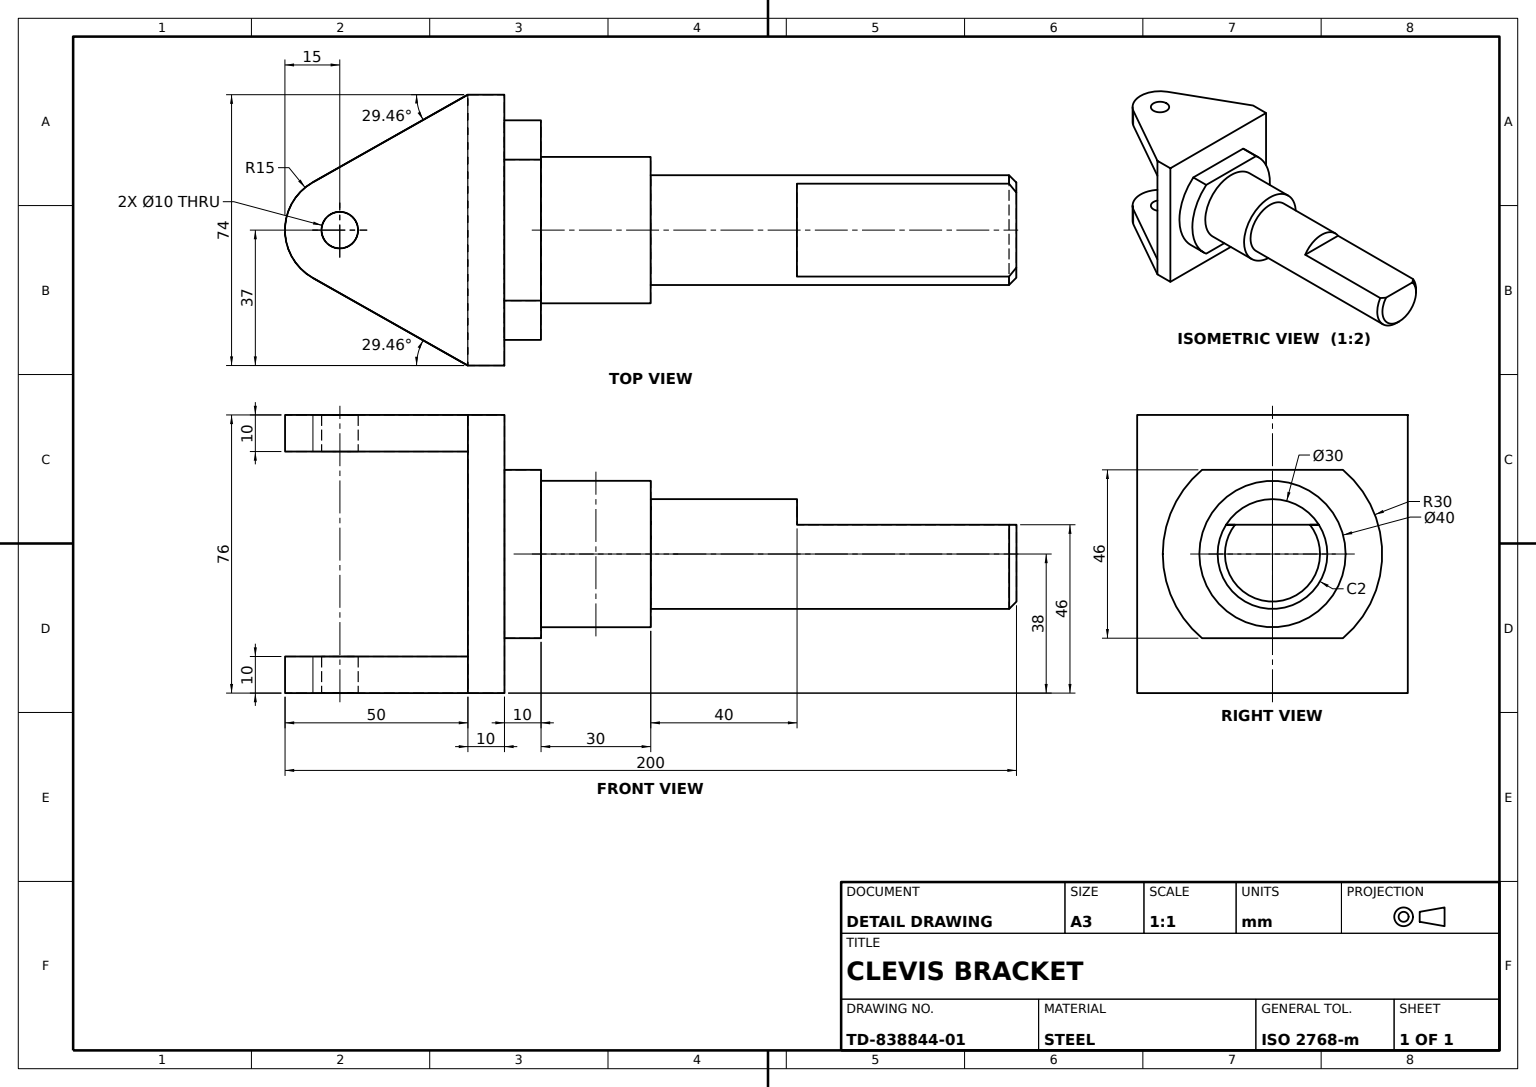
SolidWorks part; units mm, degrees
material "Plain Carbon Steel"
ref_plane "Front Plane" through (0, 0, 0) normal (0, 0, 1) x (1, 0, 0)
ref_plane "Top Plane" through (0, 0, 0) normal (0, 1, 0) x (1, 0, 0)
ref_plane "Right Plane" through (0, 0, 0) normal (1, 0, 0) x (0, 0, -1)
sketch "Base Plate Sketch" plane through (0, 0, 0) normal (0, 0, 1) x (1, 0, 0)
  line L0 (0, -38) -> (0, 38)
  line L1 (0, 38) -> (-10, 38)
  line L2 (-10, 38) -> (-10, -38)
  line L3 (-10, -38) -> (0, -38)
  point P4 (0, 0)
  dimension "D1" = 10
  dimension "D2" = 76
extrude "Base Plate" add sketch "Base Plate Sketch" against normal blind 74
sketch "Fork Ear 1 Sketch" plane through (0, 38, 0) normal (0, 1, 0) x (1, 0, 0)
  line L0 (-10, 74) -> (-10, 0)
  line L2 (-52.3779, 50.0601) -> (-10, 74)
  line L3 (-52.3779, 23.9399) -> (-10, 0)
  arc A0 (-52.3779, 50.0601) -> (-52.3779, 23.9399) centre (-45, 37) ccw
  dimension "D2" = 30
  dimension "D3" = 42.3779
  dimension "D1" = 23.9399
extrude "Fork Ear 1" add sketch "Fork Ear 1 Sketch" against normal blind 10
sketch "Fork Ear 2 Sketch" plane through (0, -38, 0) normal (0, -1, 0) x (1, 0, 0)
  line L2 (-52.3779, -23.9399) -> (-10, 0)
  line L3 (-10, 0) -> (-10, -74)
  line L4 (-10, -74) -> (-52.3779, -50.0601)
  arc A0 (-52.3779, -23.9399) -> (-52.3779, -50.0601) centre (-45, -37) ccw
  dimension "D2" = 30
  dimension "D3" = 26.1203
  dimension "D1" = 23.9399
  dimension "D4" = 42.3779
extrude "Fork Ear 2" add sketch "Fork Ear 2 Sketch" against normal blind 10
sketch "Pivot Pin Hole Sketch" plane through (0, -38, 0) normal (0, -1, 0) x (1, 0, 0)
  circle A0 centre (-45, -37) radius 5
  dimension "D1" = 10
extrude "Pivot Pin Hole Ø10" cut sketch "Pivot Pin Hole Sketch" against normal blind 100
sketch "Hex Collar Sketch" plane through (0, 0, 0) normal (1, 0, 0) x (0, 0, -1)
  line L5 (17.7386, 23) -> (56.2614, 23)
  line L6 (74, 38) -> (0, 38) construction
  line L11 (17.7386, -23) -> (56.2614, -23)
  arc A0 (17.7386, 23) -> (17.7386, -23) centre (37, 0) ccw
  arc A2 (56.2614, -23) -> (56.2614, 23) centre (37, 0) ccw
  dimension "D1" = 60
  dimension "D3" = 23
  dimension "D2" = 15
  dimension "D4" = 46
  dimension "D5" = 17.7386
extrude "Hex Collar" add sketch "Hex Collar Sketch" along normal blind 10
sketch "Shoulder Ø40 Sketch" plane through (10, 0, 0) normal (1, 0, 0) x (0, 0, -1)
  circle A0 centre (37, 0) radius 20
  dimension "D1" = 40
extrude "Shoulder Ø40" add sketch "Shoulder Ø40 Sketch" along normal blind 30
sketch "Shaft Ø30 Sketch" plane through (40, 0, 0) normal (1, 0, 0) x (0, 0, -1)
  circle A0 centre (37, 0) radius 15
  dimension "D1" = 30
extrude "Shaft Ø30" add sketch "Shaft Ø30 Sketch" along normal blind 100
sketch "Shaft Flat Sketch" plane through (140, 0, 0) normal (1, 0, 0) x (0, 0, -1)
  line L0 (24.3114, 8) -> (49.6886, 8)
  arc A0 (49.6886, 8) -> (24.3114, 8) centre (37, 0) ccw
  dimension "D2" = 30
  dimension "D1" = 25.3772
extrude "Shaft Flat" cut sketch "Shaft Flat Sketch" against normal blind 60
chamfer "Shaft End Chamfer 2x45°" distance 2 angle 45 1 edges at (140, -15, -37)
